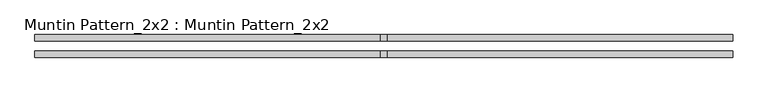
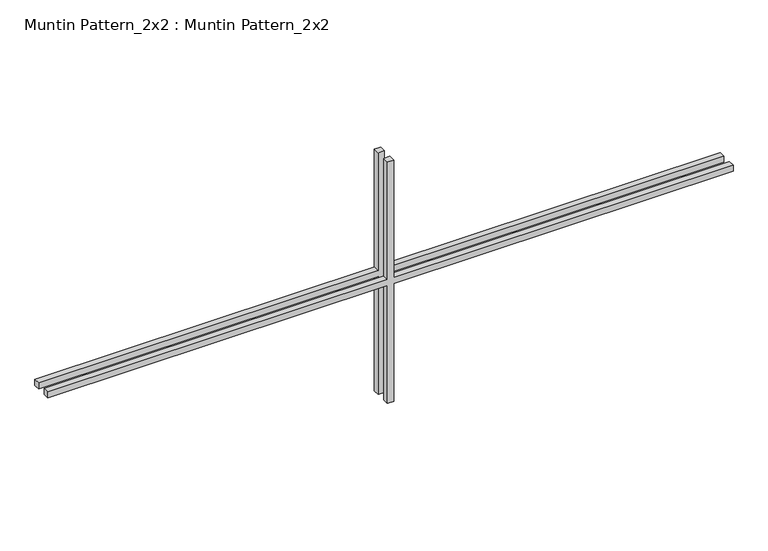
"""IFC4 building model written with IfcOpenShell, lengths in millimetres: proxy geometry, Muntin Pattern_2x2 : Muntin Pattern_2x2."""

from ifc_helpers import new_model, si_unit, frame, origin, place, context, project, spatial, polyline, outline, extrude, source, transform, mapped, element, save


def muntin_pattern_2x2_muntin_pattern_2x2_c001a7f4(model_context):
    return source(origin(), model_context, "Body", "SweptSolid", [
        extrude(outline(polyline([(261.9375, -6.35), (261.9375, -685.8), (249.2375, -685.8), (249.2375, -6.35), (0.0, -6.35), (0.0, 6.35), (249.2375, 6.35), (249.2375, 685.8), (261.9375, 685.8), (261.9375, 6.35), (511.175, 6.35), (511.175, -6.35), (261.9375, -6.35)])), frame((0.0, 9.525, 0.0), z_axis=(0.0, 1.0, 0.0), x_axis=(0.0, 0.0, 1.0)), (0.0, 0.0, 1.0), 12.7),
        extrude(outline(polyline([(261.9375, -6.35), (261.9375, -685.8), (249.2375, -685.8), (249.2375, -6.35), (0.0, -6.35), (0.0, 6.35), (249.2375, 6.35), (249.2375, 685.8), (261.9375, 685.8), (261.9375, 6.35), (511.175, 6.35), (511.175, -6.35), (261.9375, -6.35)])), frame((0.0, -22.225, 0.0), z_axis=(0.0, 1.0, 0.0), x_axis=(0.0, 0.0, 1.0)), (0.0, 0.0, 1.0), 12.7),
    ])


if __name__ == "__main__":
    model = new_model("IFC4")
    model_context = context("Model", 3, world=origin())
    ifc_project = project(units=[si_unit("LENGTHUNIT", "METRE", prefix="MILLI")], contexts=[model_context])
    site = spatial("IfcSite", under=ifc_project)
    building = spatial("IfcBuilding", under=site)
    placement = place(None, origin())
    muntin_pattern_2x2_muntin_pattern_2x2_shape = muntin_pattern_2x2_muntin_pattern_2x2_c001a7f4(model_context)
    element("IfcBuildingElementProxy", 1, Name="Muntin Pattern_2x2 : Muntin Pattern_2x2", ObjectType="Muntin Pattern_2x2 : Muntin Pattern_2x2", at=placement, inside=building, context=model_context, shape_type="MappedRepresentation", body=[
        mapped(muntin_pattern_2x2_muntin_pattern_2x2_shape, transform((0.0, 0.0, 0.0), x_axis=(1.0, 0.0, 0.0), y_axis=(0.0, 1.0, 0.0), z_axis=(0.0, 0.0, 1.0))),
    ])
    save(model, "model.ifc")

# Revit data of these elements
# Type "Muntin Pattern_2x2 : Muntin Pattern_2x2"
#   Width [instance default] = 4' - 0"
#   Thickness = 0' - 0 1/2"
#   Height [instance default] = 4' - 0"
#   Distance = 0' - 0 3/4"
#   Interior Material [instance default] = none
#   Exterior Material [instance default] = none
#   Default Elevation = 0
# Element 1 (IfcBuildingElementProxy, "Muntin Pattern_2x2 : Muntin Pattern_2x2")
#   Width = 4' - 6"
#   Height = 1' - 8 1/8"
#   Interior Material = Wood - Stained
#   Exterior Material = Clad - White
#   Materials on its faces: "Clad - White", "Wood - Stained"
# Materials
#   "Clad - White": class "Wood", colour RGB 242 242 238, transparency 0, Cost = 0
#   "Wood - Stained": class "Wood", colour RGB 224 178 126, transparency 0, Cost = 0
